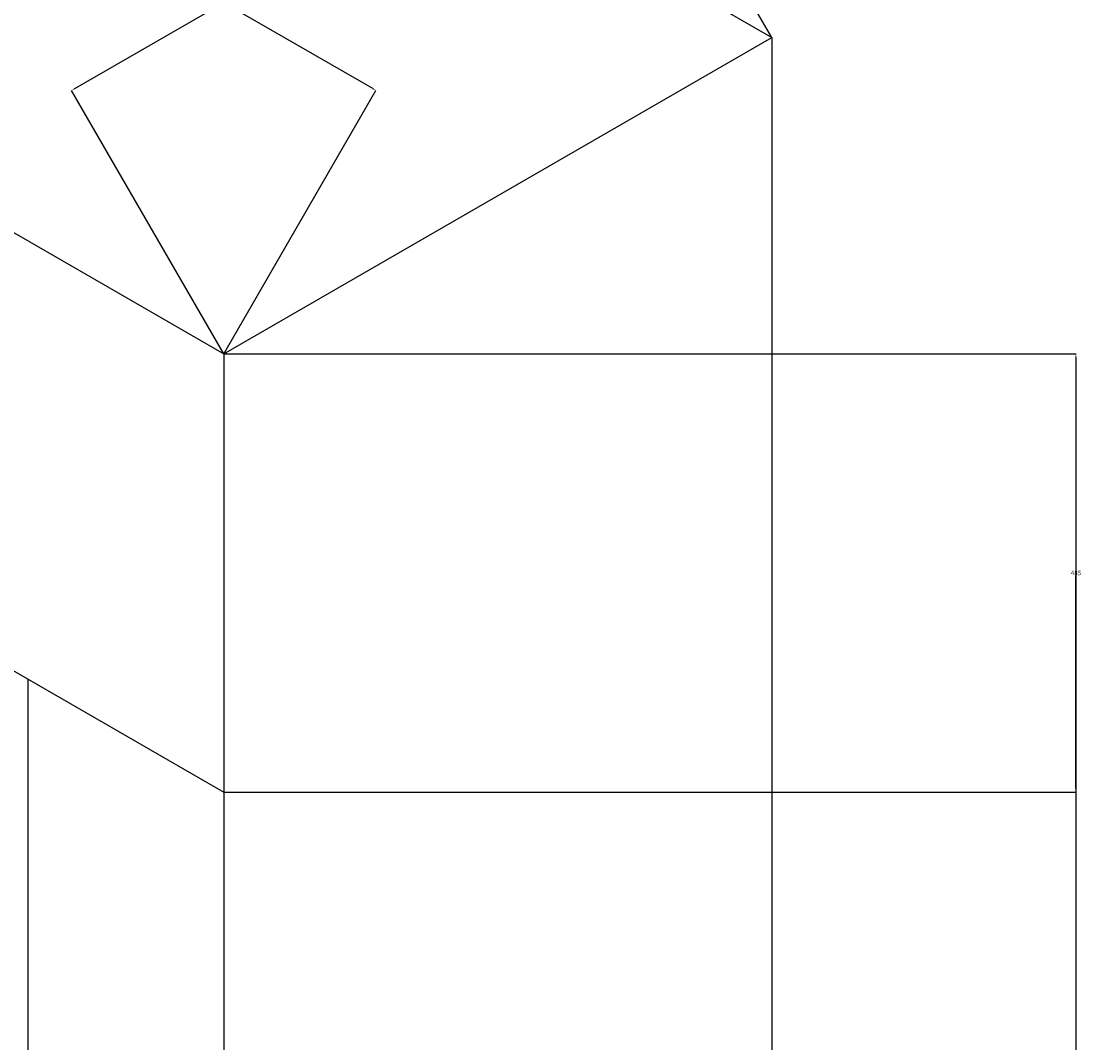
# Model space of a CAD drawing. Units: metres. Extents: x -2391 to 4922, y -635 to 4845.
# Tile 36 of 37: x 3747 to 4922, y 1238 to 2368. Entities that reach past the tile are written whole.
import ezdxf

# ---------------------------------------------------------------- set-up
doc = ezdxf.new("R2010")
doc.units = ezdxf.units.M
doc.header["$MEASUREMENT"] = 0
doc.layers.add('A-ANNO-DIMS', color=2, linetype='Continuous', lineweight=18)
doc.layers.add('A-FLOR-FIXT', color=3, linetype='Continuous', lineweight=25)
doc.styles.get("Standard").update_dxf_attribs({"font": 'arial.ttf'})
doc.dimstyles.get("Standard").update_dxf_attribs({"dimtxt": 5, "dimasz": 4, "dimexe": 0.18, "dimexo": 0.0625, "dimgap": 0.09, "dimtad": 0, "dimtih": 1, "dimtoh": 1, "dimdec": 0, "dimzin": 0, "dimdsep": 46, "dimtxsty": 'Standard', "dimcen": 0.09, "dimadec": 0, "dimazin": 0, "dimtfac": 1, "dimtdec": 0, "dimtofl": 0, "dimtmove": 0, "dimatfit": 3, "dimfxl": 1, "dimtolj": 1, "dimtzin": 0, "dimarcsym": 0})

# ---------------------------------------------------------------- blocks, each defined once
blk = doc.blocks.new('*D8')
at = {"layer": 'A-ANNO-DIMS', "color": 0, "lineweight": -2, "transparency": 16777216}
for p, q in [((-2047.3, 3005.2), (-2047.3, -631.4)), ((4577.8, 2350.2), (4577.8, -631.4)), ((-2043.3, -631.2), (1257.6, -631.2)), ((4573.8, -631.2), (1272.8, -631.2))]:
    blk.add_line(p, q, dxfattribs=at)
at = {"layer": 'A-ANNO-DIMS', "color": 0, "transparency": 16777216}
for points in [[(-2043.3, -630.6), (-2043.3, -631.9), (-2047.3, -631.2)], [(4573.8, -630.6), (4573.8, -631.9), (4577.8, -631.2)]]:
    blk.add_solid(points, dxfattribs=at)
at = {"layer": 'Defpoints', "color": 0, "transparency": 16777216}
for p in [(-2047.3, 3005.3), (4577.8, 2350.3), (4577.8, -631.2)]:
    blk.add_point(p, dxfattribs=at)
at = {"layer": 'A-ANNO-DIMS', "color": 0, "transparency": 16777216, "insert": (1265.2, -631.2), "char_height": 5, "attachment_point": 5}
blk.add_mtext('\\A1;6625', dxfattribs=at)
blk = doc.blocks.new('*D27')
at = {"layer": 'A-ANNO-DIMS', "color": 0, "lineweight": -2, "transparency": 16777216}
for p, q in [((3971.6, 2000.3), (4914.4, 2000.3)), ((4914.3, 1996.3), (4914.3, 1077.9)), ((4914.3, 154.3), (4914.3, 1072.6)), ((3971.6, 150.3), (4914.4, 150.3))]:
    blk.add_line(p, q, dxfattribs=at)
at = {"layer": 'A-ANNO-DIMS', "color": 0, "transparency": 16777216}
for points in [[(4913.6, 1996.3), (4914.9, 1996.3), (4914.3, 2000.3)], [(4913.6, 154.3), (4914.9, 154.3), (4914.3, 150.3)]]:
    blk.add_solid(points, dxfattribs=at)
at = {"layer": 'Defpoints', "color": 0, "transparency": 16777216}
for p in [(3971.5, 2000.3), (3971.5, 150.3), (4914.3, 150.3)]:
    blk.add_point(p, dxfattribs=at)
at = {"layer": 'A-ANNO-DIMS', "color": 0, "transparency": 16777216, "insert": (4914.3, 1075.3), "char_height": 5, "attachment_point": 5}
blk.add_mtext('\\A1;1850', dxfattribs=at)
blk = doc.blocks.new('*D28')
at = {"layer": 'A-ANNO-DIMS', "color": 0, "lineweight": -2, "transparency": 16777216}
for p, q in [((3148.8, 2475.3), (3317.2, 2766.8)), ((3320.5, 2764.7), (3723.9, 2531.8)), ((4136.3, 2293.7), (3733, 2526.6)), ((3971.6, 2000.3), (4139.9, 2291.8))]:
    blk.add_line(p, q, dxfattribs=at)
at = {"layer": 'A-ANNO-DIMS', "color": 0, "transparency": 16777216}
for points in [[(3320.9, 2765.3), (3320.2, 2764.1), (3317.1, 2766.7)], [(4136.7, 2294.3), (4136, 2293.1), (4139.8, 2291.7)]]:
    blk.add_solid(points, dxfattribs=at)
at = {"layer": 'Defpoints', "color": 0, "transparency": 16777216}
for p in [(3148.8, 2475.3), (4139.8, 2291.7), (3971.5, 2000.3)]:
    blk.add_point(p, dxfattribs=at)
at = {"layer": 'A-ANNO-DIMS', "color": 0, "transparency": 16777216, "insert": (3728.4, 2529.2), "char_height": 5, "attachment_point": 5}
blk.add_mtext('\\A1;950', dxfattribs=at)
blk = doc.blocks.new('*D29')
at = {"layer": 'A-ANNO-DIMS', "color": 0, "lineweight": -2, "transparency": 16777216}
for p, q in [((4406, 2639.7), (4111, 2469.3)), ((4577.7, 2350.3), (4409.4, 2641.8)), ((3806.8, 2293.7), (4101.8, 2464.1)), ((3971.5, 2000.3), (3803.2, 2291.8))]:
    blk.add_line(p, q, dxfattribs=at)
at = {"layer": 'A-ANNO-DIMS', "color": 0, "transparency": 16777216}
for points in [[(4405.7, 2640.3), (4406.4, 2639.1), (4409.5, 2641.7)], [(3806.4, 2294.3), (3807.1, 2293.1), (3803.3, 2291.7)]]:
    blk.add_solid(points, dxfattribs=at)
at = {"layer": 'Defpoints', "color": 0, "transparency": 16777216}
for p in [(4409.5, 2641.7), (4577.8, 2350.3), (3971.5, 2000.3)]:
    blk.add_point(p, dxfattribs=at)
at = {"layer": 'A-ANNO-DIMS', "color": 0, "transparency": 16777216, "insert": (4106.4, 2466.7), "char_height": 5, "attachment_point": 5}
blk.add_mtext('\\A1;700', dxfattribs=at)
blk = doc.blocks.new('*D30')
at = {"layer": 'A-ANNO-DIMS', "color": 0, "lineweight": -2, "transparency": 16777216}
for p, q in [((3971.6, 2000.3), (4914.4, 2000.3)), ((4914.3, 1996.3), (4914.3, 1760.4)), ((4914.3, 1519.3), (4914.3, 1755.1)), ((3971.6, 1515.3), (4914.4, 1515.3))]:
    blk.add_line(p, q, dxfattribs=at)
at = {"layer": 'A-ANNO-DIMS', "color": 0, "transparency": 16777216}
for points in [[(4913.6, 1996.3), (4914.9, 1996.3), (4914.3, 2000.3)], [(4913.6, 1519.3), (4914.9, 1519.3), (4914.3, 1515.3)]]:
    blk.add_solid(points, dxfattribs=at)
at = {"layer": 'Defpoints', "color": 0, "transparency": 16777216}
for p in [(3971.5, 2000.3), (3971.5, 1515.3), (4914.3, 1515.3)]:
    blk.add_point(p, dxfattribs=at)
at = {"layer": 'A-ANNO-DIMS', "color": 0, "transparency": 16777216, "insert": (4914.3, 1757.8), "char_height": 5, "attachment_point": 5}
blk.add_mtext('\\A1;485', dxfattribs=at)
blk = doc.blocks.new('*D31')
at = {"layer": 'A-ANNO-DIMS', "color": 0, "lineweight": -2, "transparency": 16777216}
for p, q in [((3971.6, 1515.3), (4914.4, 1515.3)), ((4914.3, 1511.3), (4914.3, 1185.4)), ((4914.3, 854.3), (4914.3, 1180.1)), ((3971.6, 850.3), (4914.4, 850.3))]:
    blk.add_line(p, q, dxfattribs=at)
at = {"layer": 'A-ANNO-DIMS', "color": 0, "transparency": 16777216}
for points in [[(4913.6, 1511.3), (4914.9, 1511.3), (4914.3, 1515.3)], [(4913.6, 854.3), (4914.9, 854.3), (4914.3, 850.3)]]:
    blk.add_solid(points, dxfattribs=at)
at = {"layer": 'Defpoints', "color": 0, "transparency": 16777216}
for p in [(3971.5, 1515.3), (3971.5, 850.3), (4914.3, 850.3)]:
    blk.add_point(p, dxfattribs=at)
at = {"layer": 'A-ANNO-DIMS', "color": 0, "transparency": 16777216, "insert": (4914.3, 1182.8), "char_height": 5, "attachment_point": 5}
blk.add_mtext('\\A1;665', dxfattribs=at)

msp = doc.modelspace()

# ---------------------------------------------------------------- linework, layer by layer
at = {"layer": 'A-FLOR-FIXT'}
for p, q in [((3755.0359, 2825.2763), (4577.76, 2350.2763)), ((3148.8181, 2475.2763), (3971.5422, 2000.2763)), ((3971.5422, 2000.2763), (4577.76, 2350.2763)), ((4577.76, 2350.2763), (4577.76, 500.2763)), ((3971.5422, 2000.2763), (3971.5422, 150.2763)), ((3148.8181, 1990.2763), (3971.5422, 1515.2763)), ((3755.0359, 975.2763), (3755.0359, 1640.2763))]:
    msp.add_line(p, q, dxfattribs=at)

# ---------------------------------------------------------------- dimensions: what is measured, and where the dimension line sits
at = {"layer": 'A-ANNO-DIMS'}
dim = msp.add_linear_dim(base=(4577.76, -631.2237), p1=(-2047.3343, 3005.2763), p2=(4577.76, 2350.2763), dimstyle='Standard', override={"dimdec": 0, "dimlfac": 1, "dimrnd": 0, "dimzin": 0, "dimdsep": 46, "dimlunit": 2}, dxfattribs=at)
dim.commit()
dim.dimension.update_dxf_attribs({"geometry": '*D8', "text_midpoint": (1265.2128, -631.2237)})
for base, p1, p2, angle, picture, middle in [((4139.7922, 2291.6938), (3148.8181, 2475.2763), (3971.5422, 2000.2763), 330, '*D28', (3728.4302, 2529.1938)), ((4409.51, 2641.6938), (3971.5422, 2000.2763), (4577.76, 2350.2763), 30, '*D29', (4106.4011, 2466.6938)), ((4914.26, 150.2763), (3971.5422, 2000.2763), (3971.5422, 150.2763), 90, '*D27', (4914.26, 1075.2763)), ((4914.26, 1515.2763), (3971.5422, 2000.2763), (3971.5422, 1515.2763), 90, '*D30', (4914.26, 1757.7763)), ((4914.26, 850.2763), (3971.5422, 1515.2763), (3971.5422, 850.2763), 90, '*D31', (4914.26, 1182.7763))]:
    dim = msp.add_linear_dim(base=base, p1=p1, p2=p2, angle=angle, dimstyle='Standard', override={"dimdec": 0, "dimlfac": 1, "dimrnd": 0, "dimzin": 0, "dimdsep": 46, "dimlunit": 2}, dxfattribs=at)
    dim.commit()
    dim.dimension.update_dxf_attribs({"geometry": picture, "text_midpoint": middle})

doc.saveas('drawing.dxf')
